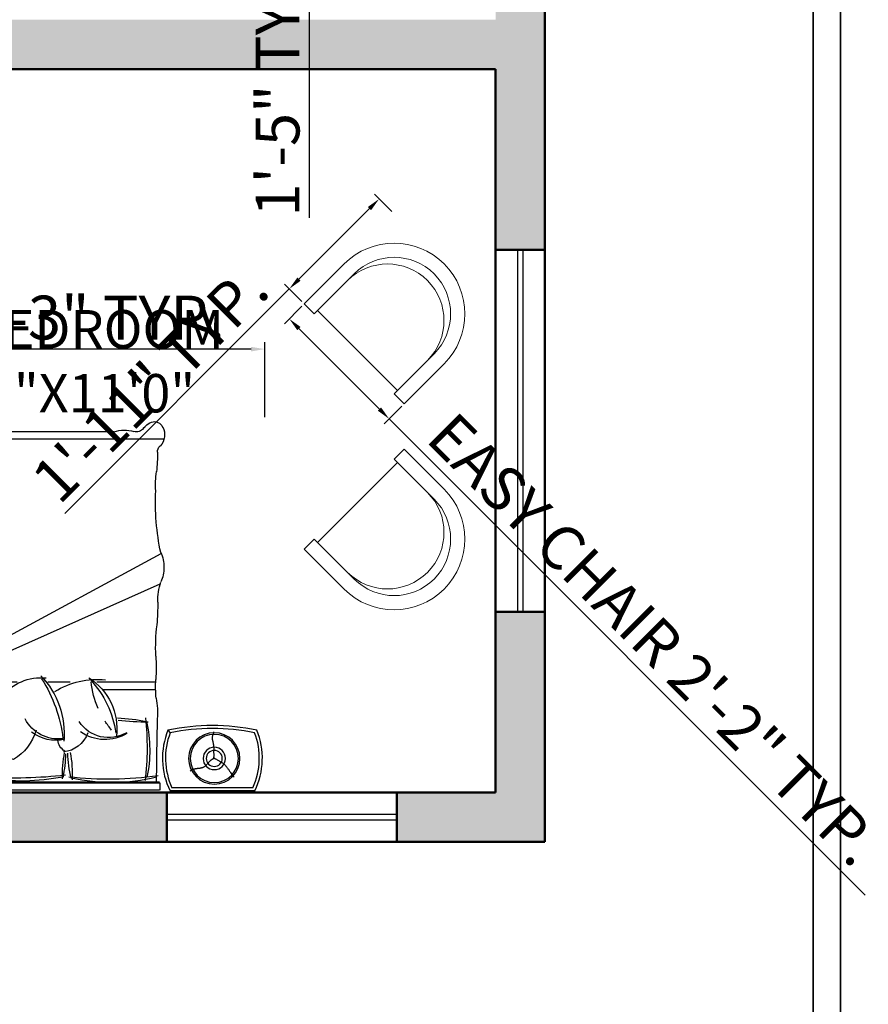
# Model space of a CAD drawing. Units: inches. Extents: x 3008 to 4088, y 1255 to 2137.
# Tile 24 of 30: x 3933 to 4088, y 1440 to 1620. Entities that reach past the tile are written whole.
import ezdxf

# ---------------------------------------------------------------- set-up
doc = ezdxf.new("R2010")
doc.units = ezdxf.units.IN
for name, color, linetype, lineweight in [('A-ANNO-DIMS', 2, 'Continuous', 18), ('A-AREA-IDEN', 7, 'Continuous', 18), ('A-FURN', 8, 'Continuous', 18), ('A-GLAZ', 4, 'Continuous', 25), ('A-WALL', 7, 'Continuous', 50), ('A-WALL-PATT', 8, 'Continuous', 13), ('C-PROP', 1, 'Continuous', 35)]:
    doc.layers.add(name, color=color, linetype=linetype, lineweight=lineweight)
doc.layers.add('TEFRİŞ', color=11, linetype='Continuous')
doc.styles.get("Standard").update_dxf_attribs({"font": 'arial.ttf'})
doc.dimstyles.new('ISO-25', dxfattribs={"dimtxt": 8, "dimasz": 2.5, "dimexe": 1.25, "dimexo": 0.625, "dimtad": 1, "dimdec": 1, "dimlunit": 3, "dimtxsty": 'Standard', "dimcen": 2.5, "dimadec": 0, "dimazin": 0, "dimtfac": 1, "dimtdec": 1, "dimtmove": 0, "dimatfit": 3, "dimfxl": 1, "dimarcsym": 0})

# ---------------------------------------------------------------- blocks, each defined once
blk = doc.blocks.new('12PSTG07')
at = {"color": 0, "linetype": 'ByBlock'}
for p, q in [((0, 15), (-12, 15)), ((0, 12), (0, 15)), ((-12, 12), (0, 12)), ((-1, -12), (-1, 12)), ((-12, -12), (0, -12)), ((0, -12), (0, -15)), ((0, -15), (-12, -15))]:
    blk.add_line(p, q, dxfattribs=at)
for centre, radius in [((-12, 0), 15), ((-12, 0), 12), ((-10, 0), 12)]:
    blk.add_arc(centre, radius, 90, 270, dxfattribs=at)
blk = doc.blocks.new('BED')
at = {"layer": 'TEFRİŞ'}
for p, q in [((2114.88, 1835.66), (2129.12, 1835.66)), ((2115.2, 1835.15), (2128.8, 1835.15)), ((2130.81, 1834.34), (2130.81, 1835.55)), ((2130.91, 1835.55), (2175.56, 1835.55)), ((2175.56, 1835.55), (2175.56, 1834.34)), ((2177.29, 1835.98), (2177.61, 1835.47)), ((2177.29, 1835.98), (2191.52, 1835.98)), ((2177.61, 1835.47), (2191.2, 1835.47)), ((2191.2, 1835.47), (2191.52, 1835.98)), ((2118.49, 1833.2), (2118.34, 1833.38)), ((2118.49, 1833.2), (2118.34, 1833.38)), ((2118.63, 1833.03), (2118.49, 1833.2)), ((2118.63, 1833.03), (2118.49, 1833.2)), ((2118.75, 1832.88), (2118.63, 1833.03)), ((2118.75, 1832.88), (2118.63, 1833.03)), ((2118.86, 1832.74), (2118.75, 1832.88)), ((2118.86, 1832.74), (2118.75, 1832.88)), ((2118.95, 1832.61), (2118.86, 1832.74)), ((2118.95, 1832.61), (2118.86, 1832.74)), ((2175.56, 1834.34), (2130.81, 1834.34)), ((2175, 1834.19), (2130.91, 1834.19)), ((2180.9, 1833.52), (2180.75, 1833.7)), ((2180.9, 1833.52), (2180.75, 1833.7)), ((2181.04, 1833.35), (2180.9, 1833.52)), ((2181.04, 1833.35), (2180.9, 1833.52)), ((2181.16, 1833.2), (2181.04, 1833.35)), ((2181.16, 1833.2), (2181.04, 1833.35)), ((2181.26, 1833.06), (2181.16, 1833.2)), ((2181.26, 1833.06), (2181.16, 1833.2)), ((2181.36, 1832.93), (2181.26, 1833.06)), ((2181.36, 1832.93), (2181.26, 1833.06)), ((2181.44, 1832.8), (2181.36, 1832.93)), ((2181.44, 1832.8), (2181.36, 1832.93)), ((2181.52, 1832.69), (2181.44, 1832.8)), ((2181.52, 1832.69), (2181.44, 1832.8)), ((2119.04, 1832.48), (2118.95, 1832.61)), ((2119.04, 1832.48), (2118.95, 1832.61)), ((2119.12, 1832.37), (2119.04, 1832.48)), ((2119.12, 1832.37), (2119.04, 1832.48)), ((2119.19, 1832.26), (2119.12, 1832.37)), ((2119.19, 1832.26), (2119.12, 1832.37)), ((2119.26, 1832.16), (2119.19, 1832.26)), ((2119.26, 1832.16), (2119.19, 1832.26)), ((2119.32, 1832.06), (2119.26, 1832.16)), ((2119.32, 1832.06), (2119.26, 1832.16)), ((2119.39, 1831.97), (2119.32, 1832.06)), ((2119.39, 1831.97), (2119.32, 1832.06)), ((2119.45, 1831.89), (2119.39, 1831.97)), ((2119.45, 1831.89), (2119.39, 1831.97)), ((2119.51, 1831.81), (2119.45, 1831.89)), ((2119.51, 1831.81), (2119.45, 1831.89)), ((2119.57, 1831.73), (2119.51, 1831.81)), ((2119.57, 1831.73), (2119.51, 1831.81)), ((2119.63, 1831.65), (2119.57, 1831.73)), ((2119.63, 1831.65), (2119.57, 1831.73)), ((2119.69, 1831.58), (2119.63, 1831.65)), ((2119.69, 1831.58), (2119.63, 1831.65)), ((2119.75, 1831.51), (2119.69, 1831.58)), ((2119.75, 1831.51), (2119.69, 1831.58)), ((2119.81, 1831.44), (2119.75, 1831.51)), ((2119.81, 1831.44), (2119.75, 1831.51)), ((2119.87, 1831.38), (2119.81, 1831.44)), ((2119.87, 1831.38), (2119.81, 1831.44)), ((2119.93, 1831.31), (2119.87, 1831.38)), ((2119.93, 1831.31), (2119.87, 1831.38)), ((2119.99, 1831.25), (2119.93, 1831.31)), ((2119.99, 1831.25), (2119.93, 1831.31)), ((2120.05, 1831.2), (2119.99, 1831.25)), ((2120.05, 1831.2), (2119.99, 1831.25)), ((2120.12, 1831.14), (2120.05, 1831.2)), ((2120.12, 1831.14), (2120.05, 1831.2)), ((2120.18, 1831.09), (2120.12, 1831.14)), ((2120.18, 1831.09), (2120.12, 1831.14)), ((2120.25, 1831.04), (2120.18, 1831.09)), ((2120.25, 1831.04), (2120.18, 1831.09)), ((2120.32, 1830.99), (2120.25, 1831.04)), ((2120.32, 1830.99), (2120.25, 1831.04)), ((2122.72, 1831.01), (2122.8, 1831.09)), ((2122.72, 1831.01), (2122.8, 1831.09)), ((2122.8, 1831.09), (2122.87, 1831.18)), ((2122.8, 1831.09), (2122.87, 1831.18)), ((2122.87, 1831.18), (2122.94, 1831.26)), ((2122.87, 1831.18), (2122.94, 1831.26)), ((2122.94, 1831.26), (2123.01, 1831.33)), ((2122.94, 1831.26), (2123.01, 1831.33)), ((2123.01, 1831.33), (2123.08, 1831.4)), ((2123.01, 1831.33), (2123.08, 1831.4)), ((2123.08, 1831.4), (2123.14, 1831.46)), ((2123.08, 1831.4), (2123.14, 1831.46)), ((2123.14, 1831.46), (2123.21, 1831.52)), ((2123.14, 1831.46), (2123.21, 1831.52)), ((2123.21, 1831.52), (2123.27, 1831.58)), ((2123.21, 1831.52), (2123.27, 1831.58)), ((2123.27, 1831.58), (2123.34, 1831.63)), ((2123.27, 1831.58), (2123.34, 1831.63)), ((2123.34, 1831.63), (2123.41, 1831.67)), ((2123.34, 1831.63), (2123.41, 1831.67)), ((2123.41, 1831.67), (2123.48, 1831.71)), ((2123.41, 1831.67), (2123.48, 1831.71)), ((2123.48, 1831.71), (2123.55, 1831.74)), ((2123.48, 1831.71), (2123.55, 1831.74)), ((2123.55, 1831.74), (2123.62, 1831.77)), ((2123.55, 1831.74), (2123.62, 1831.77)), ((2123.62, 1831.77), (2123.69, 1831.8)), ((2123.62, 1831.77), (2123.69, 1831.8)), ((2123.69, 1831.8), (2123.77, 1831.82)), ((2123.69, 1831.8), (2123.77, 1831.82)), ((2123.77, 1831.82), (2123.84, 1831.84)), ((2123.77, 1831.82), (2123.84, 1831.84)), ((2123.84, 1831.84), (2123.91, 1831.86)), ((2123.84, 1831.84), (2123.91, 1831.86)), ((2123.91, 1831.86), (2123.98, 1831.87)), ((2123.91, 1831.86), (2123.98, 1831.87)), ((2123.98, 1831.87), (2124.06, 1831.89)), ((2123.98, 1831.87), (2124.06, 1831.89)), ((2124.06, 1831.89), (2124.13, 1831.9)), ((2124.06, 1831.89), (2124.13, 1831.9)), ((2124.13, 1831.9), (2124.2, 1831.91)), ((2124.13, 1831.9), (2124.2, 1831.91)), ((2124.2, 1831.91), (2124.27, 1831.91)), ((2124.2, 1831.91), (2124.27, 1831.91)), ((2124.27, 1831.91), (2124.35, 1831.92)), ((2124.27, 1831.91), (2124.35, 1831.92)), ((2124.35, 1831.92), (2124.42, 1831.93)), ((2124.35, 1831.92), (2124.42, 1831.93)), ((2124.42, 1831.93), (2124.49, 1831.94)), ((2124.42, 1831.93), (2124.49, 1831.94)), ((2124.49, 1831.94), (2124.56, 1831.95)), ((2124.49, 1831.94), (2124.56, 1831.95)), ((2124.56, 1831.95), (2124.64, 1831.96)), ((2124.56, 1831.95), (2124.64, 1831.96)), ((2124.64, 1831.96), (2124.71, 1831.98)), ((2124.64, 1831.96), (2124.71, 1831.98)), ((2124.71, 1831.98), (2124.79, 1831.99)), ((2124.71, 1831.98), (2124.79, 1831.99)), ((2124.79, 1831.99), (2124.87, 1832.01)), ((2124.79, 1831.99), (2124.87, 1832.01)), ((2124.87, 1832.01), (2124.96, 1832.03)), ((2124.87, 1832.01), (2124.96, 1832.03)), ((2124.96, 1832.03), (2125.05, 1832.05)), ((2124.96, 1832.03), (2125.05, 1832.05)), ((2125.05, 1832.05), (2125.14, 1832.08)), ((2125.05, 1832.05), (2125.14, 1832.08)), ((2125.14, 1832.08), (2125.23, 1832.11)), ((2125.14, 1832.08), (2125.23, 1832.11)), ((2125.23, 1832.11), (2125.33, 1832.14)), ((2125.23, 1832.11), (2125.33, 1832.14)), ((2125.33, 1832.14), (2125.42, 1832.17)), ((2125.33, 1832.14), (2125.42, 1832.17)), ((2125.42, 1832.17), (2125.52, 1832.21)), ((2125.42, 1832.17), (2125.52, 1832.21)), ((2125.52, 1832.21), (2125.6, 1832.25)), ((2125.52, 1832.21), (2125.6, 1832.25)), ((2125.6, 1832.25), (2125.68, 1832.3)), ((2125.6, 1832.25), (2125.68, 1832.3)), ((2125.68, 1832.3), (2125.75, 1832.35)), ((2125.68, 1832.3), (2125.75, 1832.35)), ((2181.59, 1832.58), (2181.52, 1832.69)), ((2181.59, 1832.58), (2181.52, 1832.69)), ((2181.66, 1832.48), (2181.59, 1832.58)), ((2181.66, 1832.48), (2181.59, 1832.58)), ((2181.73, 1832.38), (2181.66, 1832.48)), ((2181.73, 1832.38), (2181.66, 1832.48)), ((2181.79, 1832.29), (2181.73, 1832.38)), ((2181.79, 1832.29), (2181.73, 1832.38)), ((2181.85, 1832.21), (2181.79, 1832.29)), ((2181.85, 1832.21), (2181.79, 1832.29)), ((2181.92, 1832.13), (2181.85, 1832.21)), ((2181.92, 1832.13), (2181.85, 1832.21)), ((2181.97, 1832.05), (2181.92, 1832.13)), ((2181.97, 1832.05), (2181.92, 1832.13)), ((2182.03, 1831.97), (2181.97, 1832.05)), ((2182.03, 1831.97), (2181.97, 1832.05)), ((2182.09, 1831.9), (2182.03, 1831.97)), ((2182.09, 1831.9), (2182.03, 1831.97)), ((2182.15, 1831.83), (2182.09, 1831.9)), ((2182.15, 1831.83), (2182.09, 1831.9)), ((2182.21, 1831.76), (2182.15, 1831.83)), ((2182.21, 1831.76), (2182.15, 1831.83)), ((2182.27, 1831.7), (2182.21, 1831.76)), ((2182.27, 1831.7), (2182.21, 1831.76)), ((2182.33, 1831.63), (2182.27, 1831.7)), ((2182.33, 1831.63), (2182.27, 1831.7)), ((2182.4, 1831.57), (2182.33, 1831.63)), ((2182.4, 1831.57), (2182.33, 1831.63)), ((2182.46, 1831.52), (2182.4, 1831.57)), ((2182.46, 1831.52), (2182.4, 1831.57)), ((2182.52, 1831.46), (2182.46, 1831.52)), ((2182.52, 1831.46), (2182.46, 1831.52)), ((2182.59, 1831.41), (2182.52, 1831.46)), ((2182.59, 1831.41), (2182.52, 1831.46)), ((2182.66, 1831.36), (2182.59, 1831.41)), ((2182.66, 1831.36), (2182.59, 1831.41)), ((2182.73, 1831.31), (2182.66, 1831.36)), ((2182.73, 1831.31), (2182.66, 1831.36)), ((2182.8, 1831.26), (2182.73, 1831.31)), ((2182.8, 1831.26), (2182.73, 1831.31)), ((2182.87, 1831.22), (2182.8, 1831.26)), ((2182.87, 1831.22), (2182.8, 1831.26)), ((2182.95, 1831.17), (2182.87, 1831.22)), ((2182.95, 1831.17), (2182.87, 1831.22)), ((2183.03, 1831.12), (2182.95, 1831.17)), ((2183.03, 1831.12), (2182.95, 1831.17)), ((2183.11, 1831.07), (2183.03, 1831.12)), ((2183.11, 1831.07), (2183.03, 1831.12)), ((2183.2, 1831.02), (2183.11, 1831.07)), ((2183.2, 1831.02), (2183.11, 1831.07)), ((2184.85, 1831.04), (2184.95, 1831.14)), ((2184.85, 1831.04), (2184.95, 1831.14)), ((2184.95, 1831.14), (2185.05, 1831.23)), ((2184.95, 1831.14), (2185.05, 1831.23)), ((2185.05, 1831.23), (2185.13, 1831.33)), ((2185.05, 1831.23), (2185.13, 1831.33)), ((2185.13, 1831.33), (2185.21, 1831.41)), ((2185.13, 1831.33), (2185.21, 1831.41)), ((2185.21, 1831.41), (2185.28, 1831.5)), ((2185.21, 1831.41), (2185.28, 1831.5)), ((2185.28, 1831.5), (2185.35, 1831.58)), ((2185.28, 1831.5), (2185.35, 1831.58)), ((2185.35, 1831.58), (2185.42, 1831.65)), ((2185.35, 1831.58), (2185.42, 1831.65)), ((2185.42, 1831.65), (2185.48, 1831.72)), ((2185.42, 1831.65), (2185.48, 1831.72)), ((2185.48, 1831.72), (2185.55, 1831.78)), ((2185.48, 1831.72), (2185.55, 1831.78)), ((2185.55, 1831.78), (2185.61, 1831.84)), ((2185.55, 1831.78), (2185.61, 1831.84)), ((2185.61, 1831.84), (2185.68, 1831.9)), ((2185.61, 1831.84), (2185.68, 1831.9)), ((2185.68, 1831.9), (2185.75, 1831.95)), ((2185.68, 1831.9), (2185.75, 1831.95)), ((2185.75, 1831.95), (2185.82, 1831.99)), ((2185.75, 1831.95), (2185.82, 1831.99)), ((2185.82, 1831.99), (2185.89, 1832.03)), ((2185.82, 1831.99), (2185.89, 1832.03)), ((2185.89, 1832.03), (2185.96, 1832.06)), ((2185.89, 1832.03), (2185.96, 1832.06)), ((2185.96, 1832.06), (2186.03, 1832.09)), ((2185.96, 1832.06), (2186.03, 1832.09)), ((2186.03, 1832.09), (2186.1, 1832.12)), ((2186.03, 1832.09), (2186.1, 1832.12)), ((2186.1, 1832.12), (2186.17, 1832.14)), ((2186.1, 1832.12), (2186.17, 1832.14)), ((2186.17, 1832.14), (2186.24, 1832.16)), ((2186.17, 1832.14), (2186.24, 1832.16)), ((2186.24, 1832.16), (2186.32, 1832.18)), ((2186.24, 1832.16), (2186.32, 1832.18)), ((2186.32, 1832.18), (2186.39, 1832.19)), ((2186.32, 1832.18), (2186.39, 1832.19)), ((2186.39, 1832.19), (2186.46, 1832.21)), ((2186.39, 1832.19), (2186.46, 1832.21)), ((2186.46, 1832.21), (2186.53, 1832.22)), ((2186.46, 1832.21), (2186.53, 1832.22)), ((2186.53, 1832.22), (2186.61, 1832.23)), ((2186.53, 1832.22), (2186.61, 1832.23)), ((2186.61, 1832.23), (2186.68, 1832.23)), ((2186.61, 1832.23), (2186.68, 1832.23)), ((2186.68, 1832.23), (2186.75, 1832.24)), ((2186.68, 1832.23), (2186.75, 1832.24)), ((2186.75, 1832.24), (2186.82, 1832.25)), ((2186.75, 1832.24), (2186.82, 1832.25)), ((2186.82, 1832.25), (2186.9, 1832.26)), ((2186.82, 1832.25), (2186.9, 1832.26)), ((2186.9, 1832.26), (2186.97, 1832.27)), ((2186.9, 1832.26), (2186.97, 1832.27)), ((2186.97, 1832.27), (2187.04, 1832.28)), ((2186.97, 1832.27), (2187.04, 1832.28)), ((2187.04, 1832.28), (2187.12, 1832.3)), ((2187.04, 1832.28), (2187.12, 1832.3)), ((2187.12, 1832.3), (2187.2, 1832.31)), ((2187.12, 1832.3), (2187.2, 1832.31)), ((2187.2, 1832.31), (2187.28, 1832.33)), ((2187.2, 1832.31), (2187.28, 1832.33)), ((2187.28, 1832.33), (2187.36, 1832.35)), ((2187.28, 1832.33), (2187.36, 1832.35)), ((2187.36, 1832.35), (2187.45, 1832.37)), ((2187.36, 1832.35), (2187.45, 1832.37)), ((2187.45, 1832.37), (2187.54, 1832.4)), ((2187.45, 1832.37), (2187.54, 1832.4)), ((2187.54, 1832.4), (2187.64, 1832.43)), ((2187.54, 1832.4), (2187.64, 1832.43)), ((2187.64, 1832.43), (2187.74, 1832.46)), ((2187.64, 1832.43), (2187.74, 1832.46)), ((2187.74, 1832.46), (2187.83, 1832.49)), ((2187.74, 1832.46), (2187.83, 1832.49)), ((2187.83, 1832.49), (2187.92, 1832.53)), ((2187.83, 1832.49), (2187.92, 1832.53)), ((2187.92, 1832.53), (2188.01, 1832.57)), ((2187.92, 1832.53), (2188.01, 1832.57)), ((2188.01, 1832.57), (2188.09, 1832.62)), ((2188.01, 1832.57), (2188.09, 1832.62)), ((2188.09, 1832.62), (2188.15, 1832.67)), ((2188.09, 1832.62), (2188.15, 1832.67)), ((2120.39, 1830.94), (2120.32, 1830.99)), ((2120.39, 1830.94), (2120.32, 1830.99)), ((2120.47, 1830.9), (2120.39, 1830.94)), ((2120.47, 1830.9), (2120.39, 1830.94)), ((2120.54, 1830.85), (2120.47, 1830.9)), ((2120.54, 1830.85), (2120.47, 1830.9)), ((2120.62, 1830.8), (2120.54, 1830.85)), ((2120.62, 1830.8), (2120.54, 1830.85)), ((2120.7, 1830.75), (2120.62, 1830.8)), ((2120.7, 1830.75), (2120.62, 1830.8)), ((2120.79, 1830.7), (2120.7, 1830.75)), ((2120.79, 1830.7), (2120.7, 1830.75)), ((2120.88, 1830.65), (2120.79, 1830.7)), ((2120.88, 1830.65), (2120.79, 1830.7)), ((2120.98, 1830.59), (2120.88, 1830.65)), ((2120.98, 1830.59), (2120.88, 1830.65)), ((2121.09, 1830.52), (2120.98, 1830.59)), ((2121.09, 1830.52), (2120.98, 1830.59)), ((2121.21, 1830.45), (2121.09, 1830.52)), ((2121.21, 1830.45), (2121.09, 1830.52)), ((2121.34, 1830.38), (2121.21, 1830.45)), ((2121.34, 1830.38), (2121.21, 1830.45)), ((2121.49, 1830.29), (2121.34, 1830.38)), ((2121.49, 1830.29), (2121.34, 1830.38)), ((2121.66, 1830.21), (2121.49, 1830.29)), ((2121.66, 1830.21), (2121.49, 1830.29)), ((2121.66, 1830.18), (2121.87, 1830.29)), ((2121.66, 1830.18), (2121.87, 1830.29)), ((2121.85, 1830.11), (2121.66, 1830.21)), ((2121.85, 1830.11), (2121.66, 1830.21)), ((2121.74, 1829.99), (2121.73, 1829.83)), ((2121.74, 1829.99), (2121.73, 1829.83)), ((2121.73, 1829.83), (2121.73, 1829.69)), ((2121.73, 1829.83), (2121.73, 1829.69)), ((2121.73, 1829.69), (2121.73, 1829.57)), ((2121.73, 1829.69), (2121.73, 1829.57)), ((2121.73, 1829.57), (2121.73, 1829.45)), ((2121.73, 1829.57), (2121.73, 1829.45)), ((2121.73, 1829.45), (2121.74, 1829.35)), ((2121.73, 1829.45), (2121.74, 1829.35)), ((2121.76, 1830.38), (2121.74, 1830.17)), ((2121.76, 1830.38), (2121.74, 1830.17)), ((2121.74, 1830.17), (2121.74, 1829.99)), ((2121.74, 1830.17), (2121.74, 1829.99)), ((2121.87, 1830.29), (2122.04, 1830.4)), ((2121.87, 1830.29), (2122.04, 1830.4)), ((2122.04, 1830.4), (2122.2, 1830.51)), ((2122.04, 1830.4), (2122.2, 1830.51)), ((2122.2, 1830.51), (2122.33, 1830.61)), ((2122.2, 1830.51), (2122.33, 1830.61)), ((2122.33, 1830.61), (2122.45, 1830.72)), ((2122.33, 1830.61), (2122.45, 1830.72)), ((2122.45, 1830.72), (2122.55, 1830.82)), ((2122.45, 1830.72), (2122.55, 1830.82)), ((2122.55, 1830.82), (2122.64, 1830.91)), ((2122.55, 1830.82), (2122.64, 1830.91)), ((2122.64, 1830.91), (2122.72, 1831.01)), ((2122.64, 1830.91), (2122.72, 1831.01)), ((2183.29, 1830.97), (2183.2, 1831.02)), ((2183.29, 1830.97), (2183.2, 1831.02)), ((2183.39, 1830.91), (2183.29, 1830.97)), ((2183.39, 1830.91), (2183.29, 1830.97)), ((2183.49, 1830.84), (2183.39, 1830.91)), ((2183.49, 1830.84), (2183.39, 1830.91)), ((2183.61, 1830.77), (2183.49, 1830.84)), ((2183.61, 1830.77), (2183.49, 1830.84)), ((2183.75, 1830.7), (2183.61, 1830.77)), ((2183.75, 1830.7), (2183.61, 1830.77)), ((2183.9, 1830.61), (2183.75, 1830.7)), ((2183.9, 1830.61), (2183.75, 1830.7)), ((2184.06, 1830.53), (2183.9, 1830.61)), ((2184.06, 1830.53), (2183.9, 1830.61)), ((2184.25, 1830.43), (2184.06, 1830.53)), ((2184.25, 1830.43), (2184.06, 1830.53)), ((2184.07, 1830.5), (2184.27, 1830.61)), ((2184.07, 1830.5), (2184.27, 1830.61)), ((2184.15, 1830.49), (2184.14, 1830.31)), ((2184.15, 1830.49), (2184.14, 1830.31)), ((2184.14, 1830.31), (2184.14, 1830.15)), ((2184.14, 1830.31), (2184.14, 1830.15)), ((2184.14, 1830.15), (2184.14, 1830.01)), ((2184.14, 1830.15), (2184.14, 1830.01)), ((2184.14, 1830.01), (2184.14, 1829.89)), ((2184.14, 1830.01), (2184.14, 1829.89)), ((2184.14, 1829.89), (2184.14, 1829.77)), ((2184.14, 1829.89), (2184.14, 1829.77)), ((2184.14, 1829.77), (2184.14, 1829.67)), ((2184.14, 1829.77), (2184.14, 1829.67)), ((2184.14, 1829.67), (2184.15, 1829.57)), ((2184.14, 1829.67), (2184.15, 1829.57)), ((2184.17, 1830.7), (2184.15, 1830.49)), ((2184.17, 1830.7), (2184.15, 1830.49)), ((2184.15, 1829.57), (2184.15, 1829.48)), ((2184.15, 1829.57), (2184.15, 1829.48)), ((2184.15, 1829.48), (2184.15, 1829.38)), ((2184.15, 1829.48), (2184.15, 1829.38)), ((2184.27, 1830.61), (2184.45, 1830.72)), ((2184.27, 1830.61), (2184.45, 1830.72)), ((2184.45, 1830.72), (2184.6, 1830.83)), ((2184.45, 1830.72), (2184.6, 1830.83)), ((2184.6, 1830.83), (2184.74, 1830.93)), ((2184.6, 1830.83), (2184.74, 1830.93)), ((2184.74, 1830.93), (2184.85, 1831.04)), ((2184.74, 1830.93), (2184.85, 1831.04)), ((2121.74, 1828.89), (2121.73, 1828.8)), ((2121.74, 1828.89), (2121.73, 1828.8)), ((2121.73, 1828.8), (2121.73, 1828.72)), ((2121.73, 1828.8), (2121.73, 1828.72)), ((2121.73, 1828.72), (2121.73, 1828.64)), ((2121.73, 1828.72), (2121.73, 1828.64)), ((2121.73, 1828.64), (2121.73, 1828.56)), ((2121.73, 1828.64), (2121.73, 1828.56)), ((2121.73, 1828.56), (2121.73, 1828.48)), ((2121.73, 1828.56), (2121.73, 1828.48)), ((2121.73, 1828.48), (2121.73, 1828.4)), ((2121.73, 1828.48), (2121.73, 1828.4)), ((2121.73, 1828.4), (2121.73, 1828.33)), ((2121.73, 1828.4), (2121.73, 1828.33)), ((2121.73, 1828.33), (2121.74, 1828.25)), ((2121.73, 1828.33), (2121.74, 1828.25)), ((2121.74, 1829.35), (2121.74, 1829.25)), ((2121.74, 1829.35), (2121.74, 1829.25)), ((2121.74, 1829.25), (2121.74, 1829.16)), ((2121.74, 1829.25), (2121.74, 1829.16)), ((2121.74, 1829.16), (2121.74, 1829.06)), ((2121.74, 1829.16), (2121.74, 1829.06)), ((2121.74, 1829.06), (2121.74, 1828.97)), ((2121.74, 1829.06), (2121.74, 1828.97)), ((2121.74, 1828.97), (2121.74, 1828.89)), ((2121.74, 1828.97), (2121.74, 1828.89)), ((2121.74, 1828.25), (2121.75, 1828.18)), ((2121.74, 1828.25), (2121.75, 1828.18)), ((2121.75, 1828.18), (2121.75, 1828.1)), ((2121.75, 1828.18), (2121.75, 1828.1)), ((2121.75, 1828.1), (2121.76, 1828.03)), ((2121.75, 1828.1), (2121.76, 1828.03)), ((2121.76, 1828.03), (2121.78, 1827.95)), ((2121.76, 1828.03), (2121.78, 1827.95)), ((2121.78, 1827.95), (2121.79, 1827.88)), ((2121.78, 1827.95), (2121.79, 1827.88)), ((2121.79, 1827.88), (2121.8, 1827.8)), ((2121.79, 1827.88), (2121.8, 1827.8)), ((2121.8, 1827.8), (2121.82, 1827.72)), ((2121.8, 1827.8), (2121.82, 1827.72)), ((2184.14, 1829.04), (2184.13, 1828.96)), ((2184.14, 1829.04), (2184.13, 1828.96)), ((2184.13, 1828.96), (2184.13, 1828.88)), ((2184.13, 1828.96), (2184.13, 1828.88)), ((2184.13, 1828.88), (2184.13, 1828.8)), ((2184.13, 1828.88), (2184.13, 1828.8)), ((2184.13, 1828.8), (2184.14, 1828.72)), ((2184.13, 1828.8), (2184.14, 1828.72)), ((2184.15, 1829.38), (2184.14, 1829.29)), ((2184.15, 1829.38), (2184.14, 1829.29)), ((2184.14, 1829.29), (2184.14, 1829.21)), ((2184.14, 1829.29), (2184.14, 1829.21)), ((2184.14, 1829.21), (2184.14, 1829.12)), ((2184.14, 1829.21), (2184.14, 1829.12)), ((2184.14, 1829.12), (2184.14, 1829.04)), ((2184.14, 1829.12), (2184.14, 1829.04)), ((2184.14, 1828.72), (2184.14, 1828.65)), ((2184.14, 1828.72), (2184.14, 1828.65)), ((2184.14, 1828.65), (2184.15, 1828.57)), ((2184.14, 1828.65), (2184.15, 1828.57)), ((2184.15, 1828.57), (2184.15, 1828.5)), ((2184.15, 1828.57), (2184.15, 1828.5)), ((2184.15, 1828.5), (2184.16, 1828.42)), ((2184.15, 1828.5), (2184.16, 1828.42)), ((2184.16, 1828.42), (2184.17, 1828.35)), ((2184.16, 1828.42), (2184.17, 1828.35)), ((2184.17, 1828.35), (2184.18, 1828.27)), ((2184.17, 1828.35), (2184.18, 1828.27)), ((2184.18, 1828.27), (2184.19, 1828.2)), ((2184.18, 1828.27), (2184.19, 1828.2)), ((2184.19, 1828.2), (2184.21, 1828.12)), ((2184.19, 1828.2), (2184.21, 1828.12)), ((2184.21, 1828.12), (2184.22, 1828.04)), ((2184.21, 1828.12), (2184.22, 1828.04)), ((2184.22, 1828.04), (2184.24, 1827.97)), ((2184.22, 1828.04), (2184.24, 1827.97)), ((2184.24, 1827.97), (2184.26, 1827.89)), ((2184.24, 1827.97), (2184.26, 1827.89)), ((2184.26, 1827.89), (2184.28, 1827.81)), ((2184.26, 1827.89), (2184.28, 1827.81)), ((2184.28, 1827.81), (2184.3, 1827.73)), ((2184.28, 1827.81), (2184.3, 1827.73)), ((2184.3, 1827.73), (2184.32, 1827.65)), ((2184.3, 1827.73), (2184.32, 1827.65)), ((2121.82, 1827.72), (2121.84, 1827.65)), ((2121.82, 1827.72), (2121.84, 1827.65)), ((2121.87, 1826.19), (2121.83, 1826.06)), ((2121.87, 1826.19), (2121.83, 1826.06)), ((2121.84, 1827.65), (2121.85, 1827.57)), ((2121.84, 1827.65), (2121.85, 1827.57)), ((2121.85, 1827.57), (2121.87, 1827.49)), ((2121.85, 1827.57), (2121.87, 1827.49)), ((2121.87, 1827.49), (2121.89, 1827.41)), ((2121.87, 1827.49), (2121.89, 1827.41)), ((2121.91, 1826.31), (2121.87, 1826.19)), ((2121.91, 1826.31), (2121.87, 1826.19)), ((2121.89, 1827.41), (2121.91, 1827.33)), ((2121.89, 1827.41), (2121.91, 1827.33)), ((2121.91, 1827.33), (2121.93, 1827.26)), ((2121.91, 1827.33), (2121.93, 1827.26)), ((2121.95, 1826.42), (2121.91, 1826.31)), ((2121.95, 1826.42), (2121.91, 1826.31)), ((2121.93, 1827.26), (2121.95, 1827.18)), ((2121.93, 1827.26), (2121.95, 1827.18)), ((2121.95, 1827.18), (2121.97, 1827.09)), ((2121.95, 1827.18), (2121.97, 1827.09)), ((2121.97, 1826.54), (2121.95, 1826.42)), ((2121.97, 1826.54), (2121.95, 1826.42)), ((2121.97, 1827.09), (2121.99, 1827.01)), ((2121.97, 1827.09), (2121.99, 1827.01)), ((2121.99, 1826.64), (2121.97, 1826.54)), ((2121.99, 1826.64), (2121.97, 1826.54)), ((2121.99, 1827.01), (2122, 1826.93)), ((2121.99, 1827.01), (2122, 1826.93)), ((2122, 1826.74), (2121.99, 1826.64)), ((2122, 1826.74), (2121.99, 1826.64)), ((2122, 1826.93), (2122.01, 1826.84)), ((2122, 1826.93), (2122.01, 1826.84)), ((2122.01, 1826.84), (2122, 1826.74)), ((2122.01, 1826.84), (2122, 1826.74)), ((2176.94, 1825.81), (2177.31, 1826.25)), ((2184.19, 1826.25), (2184.14, 1826.12)), ((2184.19, 1826.25), (2184.14, 1826.12)), ((2184.23, 1826.38), (2184.19, 1826.25)), ((2184.23, 1826.38), (2184.19, 1826.25)), ((2184.28, 1826.51), (2184.23, 1826.38)), ((2184.28, 1826.51), (2184.23, 1826.38)), ((2184.32, 1826.63), (2184.28, 1826.51)), ((2184.32, 1826.63), (2184.28, 1826.51)), ((2184.32, 1827.65), (2184.34, 1827.58)), ((2184.32, 1827.65), (2184.34, 1827.58)), ((2184.35, 1826.74), (2184.32, 1826.63)), ((2184.35, 1826.74), (2184.32, 1826.63)), ((2184.34, 1827.58), (2184.36, 1827.5)), ((2184.34, 1827.58), (2184.36, 1827.5)), ((2184.38, 1826.86), (2184.35, 1826.74)), ((2184.38, 1826.86), (2184.35, 1826.74)), ((2184.36, 1827.5), (2184.38, 1827.41)), ((2184.36, 1827.5), (2184.38, 1827.41)), ((2184.38, 1827.41), (2184.4, 1827.33)), ((2184.38, 1827.41), (2184.4, 1827.33)), ((2184.4, 1826.96), (2184.38, 1826.86)), ((2184.4, 1826.96), (2184.38, 1826.86)), ((2184.4, 1827.33), (2184.41, 1827.25)), ((2184.4, 1827.33), (2184.41, 1827.25)), ((2184.41, 1827.06), (2184.4, 1826.96)), ((2184.41, 1827.06), (2184.4, 1826.96)), ((2184.41, 1827.25), (2184.41, 1827.16)), ((2184.41, 1827.25), (2184.41, 1827.16)), ((2184.41, 1827.16), (2184.41, 1827.06)), ((2184.41, 1827.16), (2184.41, 1827.06)), ((2191.87, 1825.81), (2191.5, 1826.25)), ((2121.78, 1825.93), (2121.74, 1825.8)), ((2121.78, 1825.93), (2121.74, 1825.8)), ((2121.83, 1826.06), (2121.78, 1825.93)), ((2121.83, 1826.06), (2121.78, 1825.93)), ((2129.46, 1825.49), (2129.09, 1825.93)), ((2174.77, 1819.77), (2130.6, 1795.83)), ((2174.77, 1820.53), (2130.76, 1800.91)), ((2140.43, 1818.69), (2131.53, 1818.69)), ((2157.71, 1818.69), (2156.77, 1818.69)), ((2170.41, 1818.69), (2164.92, 1818.69)), ((2141.43, 1817.4), (2131.53, 1817.4)), ((2149.62, 1817.4), (2145.88, 1817.4)), ((2167.36, 1817.4), (2154.77, 1817.4)), ((2175, 1776.57), (2130.11, 1776.57)), ((2138.52, 1775.41), (2167.39, 1775.41))]:
    blk.add_line(p, q, dxfattribs=at)
for centre, radius, start, end in [((2126, 1830.19), 12.39, 153.8162, 202.314), ((2126, 1830.19), 11.88, 155.3335, 201.0157), ((2118, 1830.19), 11.88, 338.9843, 24.6665), ((2118, 1830.19), 12.39, 337.686, 26.1838), ((2188.4, 1830.51), 12.39, 153.8162, 202.314), ((2188.4, 1830.51), 11.88, 155.3335, 201.0157), ((2180.41, 1830.51), 11.88, 338.9843, 24.6665), ((2180.41, 1830.51), 12.39, 337.686, 26.1838), ((2184.41, 1861.67), 36.12, 258.6773, 281.3227), ((2122, 1861.35), 36.63, 258.2443, 281.7557), ((2122, 1861.35), 36.12, 258.6773, 281.3227), ((2184.41, 1861.67), 36.63, 258.2443, 281.7557)]:
    blk.add_arc(centre, radius, start, end, dxfattribs=at)
at = {"layer": 'TEFRİŞ', "extrusion": (0, 0, -1)}
for centre, major_axis, ratio, start_param, end_param in [((2121.68, 1830.24), (-3.05, -3.05), 1, 3.926991, 10.210176), ((2121.68, 1830.24), (2.86, -2.86), 1, 5.497787, 11.780972), ((2121.68, 1830.24), (2.86, -2.86), 1, 5.497787, 11.780972), ((2138.85, 1803.05), (-22.1, 22.1), 1, 0.544604, 1.006234), ((2167.6, 1797.72), (-0.51, 36.47), 0.865194, -0.185965, 0.185965), ((2184.09, 1830.56), (-3.05, -3.05), 1, 3.926991, 10.210176), ((2184.09, 1830.56), (2.86, -2.86), 1, 5.497787, 11.780972), ((2184.09, 1830.56), (2.86, -2.86), 1, 5.497787, 11.780972), ((2139.43, 1773.84), (-42.35, 42.35), 1, 0.646251, 0.896949), ((2206.14, 1830.73), (-52.86, -52.86), 1, 0.767743, 0.83177), ((2154.7, 1828.89), (-15.68, 15.68), 1, -1.00675, -0.580436), ((2181.61, 1828.44), (-34.39, 34.39), 1, -0.888486, -0.672463), ((2164.51, 1832.79), (-13.41, 13.41), 1, -0.974476, -0.730892), ((2127.6, 1828.81), (-13.23, 13.23), 1, 2.100388, 2.328052), ((2155, 1761.9), (-50.65, -50.65), 1, 2.239512, 2.426533), ((2172.01, 1828.66), (-17.93, 17.93), 1, -0.753394, -0.598744), ((2128.44, 1832.96), (-13.26, -13.26), 1, 3.889049, 4.127298), ((2154.12, 1796.61), (-26.46, 26.46), 1, 0.596409, 0.940188), ((2183.72, 1833.22), (-17, 17), 1, -0.967105, -0.749712), ((2134, 1828.8), (-18.62, 18.62), 1, 2.173461, 2.355043), ((2168.35, 1789.27), (-1.33, 44.62), 0.875277, -0.163954, 0.163954), ((2199.2, 1828.45), (-27.06, -27.06), 1, 0.770625, 0.917228), ((2087.32, 1833.96), (-52.37, 52.37), 1, 2.358049, 2.431787), ((2164.15, 1828.7), (-6.99, 6.99), 1, 1.789136, 2.946702), ((2156.76, 1828.98), (-11.9, -11.9), 1, 3.646453, 4.226155), ((2099.77, 1830.73), (-52.86, 52.86), 1, 2.311571, 2.373849), ((2121.68, 1830.24), (1.33, -1.33), 1, 5.497787, 11.780972), ((2121.68, 1830.24), (1.33, -1.33), 1, 5.497787, 11.780972), ((2121.68, 1830.24), (0.952, -0.952), 1, 5.497787, 11.780972), ((2121.68, 1830.24), (0.952, -0.952), 1, 5.497787, 11.780972), ((2184.09, 1830.56), (1.33, -1.33), 1, 5.497787, 11.780972), ((2184.09, 1830.56), (1.33, -1.33), 1, 5.497787, 11.780972), ((2184.09, 1830.56), (0.952, -0.952), 1, 5.497787, 11.780972), ((2184.09, 1830.56), (0.952, -0.952), 1, 5.497787, 11.780972), ((2675.38, 1815.09), (-384.79, -384.79), 1, 0.80103, 0.811711), ((2159.55, 1823.33), (-5.81, 5.81), 1, -0.516587, 0.256776), ((2154.84, 1827.75), (-1.93, 1.93), 1, 0.997904, 1.977819), ((2166.67, 1824.96), (-2.93, 3.91), 0.760601, -0.723751, 0.723751), ((2153.88, 1825.05), (-9.22, 9.22), 1, 1.994956, 2.818753), ((1630.53, 1815.09), (-384.79, 384.79), 1, 2.329881, 2.340562), ((2147.44, 1824.41), (-3.36, -3.36), 1, 1.11934, 2.270556), ((2145.66, 1827.01), (-1.62, 1.62), 1, 1.310976, 2.284591), ((2172, 1826.44), (-11.23, 11.23), 1, -1.332486, -0.624868), ((2158.82, 1823.55), (-3.74, -3.74), 1, 1.730792, 3.47045), ((2141.71, 1819.83), (-11.86, 11.86), 1, 1.850844, 2.42862), ((2157.83, 1821.53), (-4.47, 4.47), 1, 0.576679, 2.021689), ((2140.05, 1819.86), (-5.1, 5.1), 1, 0.238357, 1.390139), ((2139.42, 1820.79), (-4.21, -4.21), 1, 1.82161, 3.349145), ((2148.15, 1825.25), (-7.14, -7.14), 1, 6.061986, 7.190757), ((2160.6, 1825.98), (-9.68, -9.68), 1, 0.009196, 0.886853), ((2148.35, 1820.65), (-4.63, -4.63), 1, 2.117602, 3.020837), ((2147.86, 1820.64), (-4.48, 4.48), 1, 0.665914, 1.867503), ((2170.68, 1829.67), (-16.79, 16.79), 1, -1.354718, -0.902276), ((2154.93, 1828.48), (-11.96, 11.96), 1, -1.530302, -0.934407), ((2127.37, 1815.76), (-10.68, 10.68), 1, 1.657204, 1.779381), ((2146.08, 1822.57), (-10.5, 10.5), 1, -0.951783, -0.716225), ((2132.43, 1774.09), (-35.41, -35.41), 1, 2.362911, 2.464592), ((2140.17, 1862.96), (-27.99, 27.99), 1, 3.983025, 4.107469), ((2165.73, 1860.69), (-26.41, -26.41), 1, 5.306413, 5.463767), ((2199.62, 1529.47), (-209.2, 209.2), 1, 0.675361, 0.697001), ((2159.82, 1822.57), (-10.5, -10.5), 1, 3.857817, 4.093375), ((2127.37, 1815.76), (-10.68, 10.68), 1, 1.94252, 2.248924), ((2111.06, 1818.12), (-14.48, 14.48), 1, 2.258605, 2.412359), ((2150.79, 1825.18), (-6, 6), 1, 3.032122, 4.026148), ((2159.02, 1834.9), (-3.04, 16.53), 0.830169, 2.822117, 3.461068), ((2194.85, 1818.12), (-14.48, 14.48), 1, -0.841563, -0.687809), ((2141.33, 1830.48), (-9.55, -9.55), 1, 4.941413, 5.601673), ((2169.92, 1815.01), (-27.2, -27.2), 1, 0.734393, 0.836404), ((2135.98, 1815.01), (-27.2, -27.2), 1, 3.875985, 3.977996), ((2098.24, 1811.68), (-23.54, -23.54), 1, 3.885834, 4.043401), ((2207.66, 1811.68), (-23.54, -23.54), 1, 0.668988, 0.826555), ((2189.03, 1803.74), (-40.91, -40.91), 1, 0.789771, 0.855756), ((2116.87, 1803.74), (-40.91, 40.91), 1, 2.285836, 2.351822), ((2122.14, 1803.63), (-6.39, -6.39), 1, 3.886359, 4.265474), ((2222.76, 1798.77), (-34.16, -34.16), 1, 0.743488, 0.893627), ((2135.02, 1798.41), (-3.45, 3.45), 1, -0.831635, -0.314979), ((2135.48, 1798), (-3.77, -3.77), 1, 0.329385, 0.820948), ((2148.06, 1790.38), (-0.75, 67.37), 0.394952, 1.480524, 1.661068), ((2127.76, 1790.23), (-1, 12.37), 0.296708, 1.141067, 2.000525), ((2118.49, 1784.2), (-9.24, -9.24), 1, 3.839645, 4.088086), ((2182.27, 1782.99), (-5.52, -5.52), 1, 0.671703, 0.993321), ((2162.12, 1778.86), (-21.85, 21.85), 1, -0.78611, -0.680117), ((2143.78, 1778.86), (-21.85, 21.85), 1, 2.250913, 2.356906), ((2129.83, 1778.8), (-0.986, 0.986), 1, 2.330985, 3.163296), ((2176.08, 1778.8), (-0.986, 0.986), 1, 4.690686, 5.522997), ((2132.72, 1775.92), (-1.91, -1.91), 1, 0.284117, 1.557111), ((2173.18, 1775.92), (-1.91, -1.91), 1, 3.155278, 4.428271), ((2134.73, 1774.06), (-0.964, -0.964), 1, 1.381176, 2.701227), ((2136.75, 1781.14), (-4.24, 4.24), 1, 3.62713, 4.188813), ((2169.16, 1781.14), (-4.24, 4.24), 1, 3.665169, 4.226852), ((2171.17, 1774.06), (-0.964, -0.964), 1, 2.011162, 3.331212), ((2131.79, 1775.28), (-1.11, 1.11), 1, 3.629269, 5.067473), ((2130.83, 1777), (-2.49, -2.49), 1, 4.590984, 5.084038), ((2175.07, 1777), (-2.49, 2.49), 1, 4.34074, 4.833793), ((2174.12, 1775.28), (-1.11, 1.11), 1, 2.786508, 4.224712)]:
    blk.add_ellipse(centre, major_axis=major_axis, ratio=ratio, start_param=start_param, end_param=end_param, dxfattribs=at)
blk = doc.blocks.new('*D37')
at = {"layer": 'A-ANNO-DIMS', "color": 0, "lineweight": -2, "transparency": 16777216}
for p, q in [((3890.84, 1547.21), (3890.84, 1560.88)), ((3977.82, 1547.21), (3977.82, 1560.88)), ((3975.32, 1559.63), (3893.34, 1559.63))]:
    blk.add_line(p, q, dxfattribs=at)
at = {"layer": 'A-ANNO-DIMS', "color": 0, "transparency": 16777216}
for points in [[(3893.34, 1560.04), (3893.34, 1559.21), (3890.84, 1559.63)], [(3975.32, 1560.04), (3975.32, 1559.21), (3977.82, 1559.63)]]:
    blk.add_solid(points, dxfattribs=at)
at = {"layer": 'Defpoints', "color": 0, "transparency": 16777216}
for p in [(3890.84, 1559.63), (3890.84, 1546.58), (3977.82, 1546.58)]:
    blk.add_point(p, dxfattribs=at)
at = {"layer": 'A-ANNO-DIMS', "color": 0, "transparency": 16777216, "insert": (3934.33, 1564.34), "char_height": 8, "attachment_point": 5}
blk.add_mtext('BED 7\'-3" TYP.', dxfattribs=at)
blk = doc.blocks.new('*D46')
at = {"layer": 'A-ANNO-DIMS', "color": 0, "lineweight": -2, "transparency": 16777216}
for p, q in [((3989.71, 1652.12), (3984.64, 1652.12)), ((3985.89, 1649.62), (3985.89, 1637.82)), ((3989.71, 1635.32), (3984.64, 1635.32)), ((3985.89, 1635.32), (3985.89, 1583.56))]:
    blk.add_line(p, q, dxfattribs=at)
at = {"layer": 'A-ANNO-DIMS', "color": 0, "transparency": 16777216}
for points in [[(3985.48, 1649.62), (3986.31, 1649.62), (3985.89, 1652.12)], [(3985.48, 1637.82), (3986.31, 1637.82), (3985.89, 1635.32)]]:
    blk.add_solid(points, dxfattribs=at)
at = {"layer": 'Defpoints', "color": 0, "transparency": 16777216}
for p in [(3990.33, 1652.12), (3985.89, 1635.32), (3990.33, 1635.32)]:
    blk.add_point(p, dxfattribs=at)
at = {"layer": 'A-ANNO-DIMS', "color": 0, "transparency": 16777216, "insert": (3981.18, 1608.19), "char_height": 8, "attachment_point": 5, "rotation": 90}
blk.add_mtext('1\'-5" TYP.', dxfattribs=at)
blk = doc.blocks.new('*D49')
at = {"layer": 'A-ANNO-DIMS', "color": 0, "lineweight": -2, "transparency": 16777216}
for p, q in [((3984.57, 1567.44), (3981.4, 1564.26)), ((3984.05, 1563.37), (3998.75, 1548.67)), ((4002.81, 1549.2), (3999.63, 1546.02)), ((4000.52, 1546.9), (4087.42, 1460))]:
    blk.add_line(p, q, dxfattribs=at)
at = {"layer": 'A-ANNO-DIMS', "color": 0, "transparency": 16777216}
for points in [[(3984.34, 1563.67), (3983.75, 1563.08), (3982.28, 1565.14)], [(3999.05, 1548.97), (3998.46, 1548.38), (4000.52, 1546.9)]]:
    blk.add_solid(points, dxfattribs=at)
at = {"layer": 'Defpoints', "color": 0, "transparency": 16777216}
for p in [(3985.02, 1567.88), (4003.25, 1549.64), (4000.52, 1546.9)]:
    blk.add_point(p, dxfattribs=at)
at = {"layer": 'A-ANNO-DIMS', "color": 0, "transparency": 16777216, "insert": (4048.22, 1505.94), "char_height": 8, "attachment_point": 5, "rotation": 315}
blk.add_mtext('EASY CHAIR 2\'-2" TYP.', dxfattribs=at)
blk = doc.blocks.new('*D50')
at = {"layer": 'A-ANNO-DIMS', "color": 0, "lineweight": -2, "transparency": 16777216}
for p, q in [((4000.99, 1584.73), (3997.81, 1587.91)), ((3996.93, 1585.26), (3984.05, 1572.38)), ((3982.28, 1570.61), (3941.28, 1529.62)), ((3984.57, 1568.32), (3981.4, 1571.5))]:
    blk.add_line(p, q, dxfattribs=at)
at = {"layer": 'A-ANNO-DIMS', "color": 0, "transparency": 16777216}
for points in [[(3996.63, 1585.56), (3997.22, 1584.97), (3998.69, 1587.03)], [(3983.75, 1572.68), (3984.34, 1572.09), (3982.28, 1570.61)]]:
    blk.add_solid(points, dxfattribs=at)
at = {"layer": 'Defpoints', "color": 0, "transparency": 16777216}
for p in [(4001.43, 1584.29), (3982.28, 1570.61), (3985.02, 1567.88)]:
    blk.add_point(p, dxfattribs=at)
at = {"layer": 'A-ANNO-DIMS', "color": 0, "transparency": 16777216, "insert": (3957.61, 1552.52), "char_height": 8, "attachment_point": 5, "rotation": 45}
blk.add_mtext('1\'-11" TYP.', dxfattribs=at)

msp = doc.modelspace()

# ---------------------------------------------------------------- hatches: boundary and pattern name
at = {"layer": 'A-WALL-PATT'}
h = msp.add_hatch(color=256, dxfattribs=at)
h.dxf.hatch_style = 1
h.paths.add_polyline_path([(3665.94, 1631.72), (3656.94, 1631.72), (3656.94, 1546.72), (3665.94, 1546.72)])
h.paths.add_polyline_path([(3851.94, 1619.72), (3701.94, 1619.72), (3701.94, 1610.72), (3788.94, 1610.72), (3788.94, 1469.72), (3809.94, 1469.72), (3809.94, 1478.72), (3797.94, 1478.72), (3797.94, 1550.72), (3815.94, 1550.72), (3815.94, 1556.72), (3797.94, 1556.72), (3797.94, 1610.72), (3845.94, 1610.72), (3845.94, 1586.72), (3851.94, 1586.72)])
h.paths.add_polyline_path([(4028.94, 1631.72), (4019.94, 1631.72), (4019.94, 1619.72), (3887.94, 1619.72), (3887.94, 1610.72), (4019.94, 1610.72), (4019.94, 1577.72), (4028.94, 1577.72)])
h.paths.add_polyline_path([(3875.94, 1478.72), (3851.94, 1478.72), (3851.94, 1556.72), (3845.94, 1556.72), (3845.94, 1526.72), (3845.94, 1478.72), (3833.94, 1478.72), (3833.94, 1469.72), (3875.94, 1469.72)])
h.paths.add_polyline_path([(3959.94, 1478.72), (3917.94, 1478.72), (3917.94, 1469.72), (3959.94, 1469.72)])
h.paths.add_polyline_path([(4028.94, 1511.72), (4019.94, 1511.72), (4019.94, 1478.72), (4001.94, 1478.72), (4001.94, 1469.72), (4028.94, 1469.72)])
h.paths.add_polyline_path([(4028.94, 1699.22), (4019.94, 1699.22), (4019.94, 1673.72), (3893.94, 1673.72), (3893.94, 1649.72), (3899.94, 1649.72), (3899.94, 1667.72), (4019.94, 1667.72), (4019.94, 1655.72), (4028.94, 1655.72)])
h.paths.add_polyline_path([(4028.94, 1847.72), (4019.94, 1847.72), (4019.94, 1796.72), (3863.94, 1796.72), (3863.94, 1790.72), (4019.94, 1790.72), (4019.94, 1765.22), (4028.94, 1765.22)])
h.paths.add_polyline_path([(3815.94, 1796.72), (3779.94, 1796.72), (3665.94, 1796.72), (3665.94, 1898.72), (3656.94, 1898.72), (3656.94, 1673.72), (3665.94, 1673.72), (3665.94, 1790.72), (3815.94, 1790.72)])
h.paths.add_polyline_path([(3755.94, 1949.72), (3656.94, 1949.72), (3656.94, 1940.72), (3665.94, 1940.72), (3755.94, 1940.72)])
h.paths.add_polyline_path([(3827.94, 1949.72), (3797.94, 1949.72), (3797.94, 1940.72), (3809.94, 1940.72), (3809.94, 1874.72), (3815.94, 1874.72), (3815.94, 1940.72), (3827.94, 1940.72)])
h.paths.add_polyline_path([(3953.94, 1949.72), (3851.94, 1949.72), (3851.94, 1940.72), (3863.94, 1940.72), (3863.94, 1844.72), (3809.94, 1844.72), (3809.94, 1832.72), (3815.94, 1832.72), (3815.94, 1838.72), (3863.94, 1838.72), (3869.94, 1838.72), (3869.94, 1940.72), (3953.94, 1940.72)])
h.paths.add_polyline_path([(4028.94, 1949.72), (3995.94, 1949.72), (3995.94, 1940.72), (4019.94, 1940.72), (4019.94, 1889.72), (4028.94, 1889.72)])

# ---------------------------------------------------------------- linework, layer by layer
at = {"layer": 'A-GLAZ'}
for p, q in [((4023.94, 1577.72), (4023.94, 1511.72)), ((4023.94, 1577.72), (4023.94, 1511.72)), ((4024.94, 1577.72), (4024.94, 1511.72)), ((4001.94, 1474.72), (3959.94, 1474.72)), ((4001.94, 1473.72), (3959.94, 1473.72))]:
    msp.add_line(p, q, dxfattribs=at)
at = {"layer": 'A-WALL'}
for p, q in [((4028.94, 1949.72), (4028.94, 1469.72)), ((3887.94, 1610.72), (4019.94, 1610.72)), ((4019.94, 1610.72), (4019.94, 1478.72)), ((4019.94, 1577.72), (4028.94, 1577.72)), ((4019.94, 1511.72), (4028.94, 1511.72)), ((4019.94, 1478.72), (3851.94, 1478.72)), ((3959.94, 1469.72), (3959.94, 1478.72)), ((4001.94, 1469.72), (4001.94, 1478.72)), ((4028.94, 1469.72), (3788.94, 1469.72))]:
    msp.add_line(p, q, dxfattribs=at)
at = {"layer": 'C-PROP'}
for p, q in [((4082.94, 2009.72), (4082.94, 1349.72)), ((4077.94, 2004.72), (4077.94, 1354.72))]:
    msp.add_line(p, q, dxfattribs=at)

# ---------------------------------------------------------------- block references
at = {"layer": 'A-FURN'}
for name, p, xscale, yscale, zscale, rotation in [('12PSTG07', (3994.13, 1558.76), 0.8597921787217943, 0.8597921787217943, 0.8597921787217943, 225), ('BED', (6274.6, 3474.2), 1.086875874800008, 1.086875874800008, 1.086875874800008, 180), ('12PSTG07', (3994.13, 1532.27), -0.8597921787217945, 0.8597921787217943, 0.8597921787217943, 315)]:
    msp.add_blockref(name, p, dxfattribs=dict(at, xscale=xscale, yscale=yscale, zscale=zscale, rotation=rotation))

# ---------------------------------------------------------------- texts
at = {"layer": 'A-AREA-IDEN', "insert": (3913.46, 1566.75), "char_height": 7, "attachment_point": 1}
msp.add_mtext_dynamic_manual_height_columns('{\\fTimes New Roman|b0|i0|c0|p18;M.BEDROOM\\P14\'0"X11\'0"}', width=105.6127, gutter_width=12.5, heights=[0], dxfattribs=at)

# ---------------------------------------------------------------- dimensions: what is measured, and where the dimension line sits
at = {"layer": 'A-ANNO-DIMS'}
for base, p1, p2, angle, text, picture, middle in [((3985.89, 1635.32), (3990.33, 1652.12), (3990.33, 1635.32), 270, '<> TYP.', '*D46', (3981.18, 1608.19)), ((3982.28, 1570.61), (4001.43, 1584.29), (3985.02, 1567.88), 225, '<> TYP.', '*D50', (3957.61, 1552.52)), ((3890.84, 1559.63), (3977.82, 1546.58), (3890.84, 1546.58), 180, 'BED <> TYP.', '*D37', (3934.33, 1564.34)), ((4000.52, 1546.9), (3985.02, 1567.88), (4003.25, 1549.64), 315, 'EASY CHAIR <> TYP.', '*D49', (4048.22, 1505.94))]:
    dim = msp.add_linear_dim(base=base, p1=p1, p2=p2, angle=angle, text=text, dimstyle='ISO-25', override={"dimdec": 1, "dimrnd": 0, "dimzin": 1, "dimlunit": 4, "dimfrac": 2}, dxfattribs=at)
    dim.commit()
    dim.dimension.update_dxf_attribs({"geometry": picture, "text_midpoint": middle})

doc.saveas('drawing.dxf')
